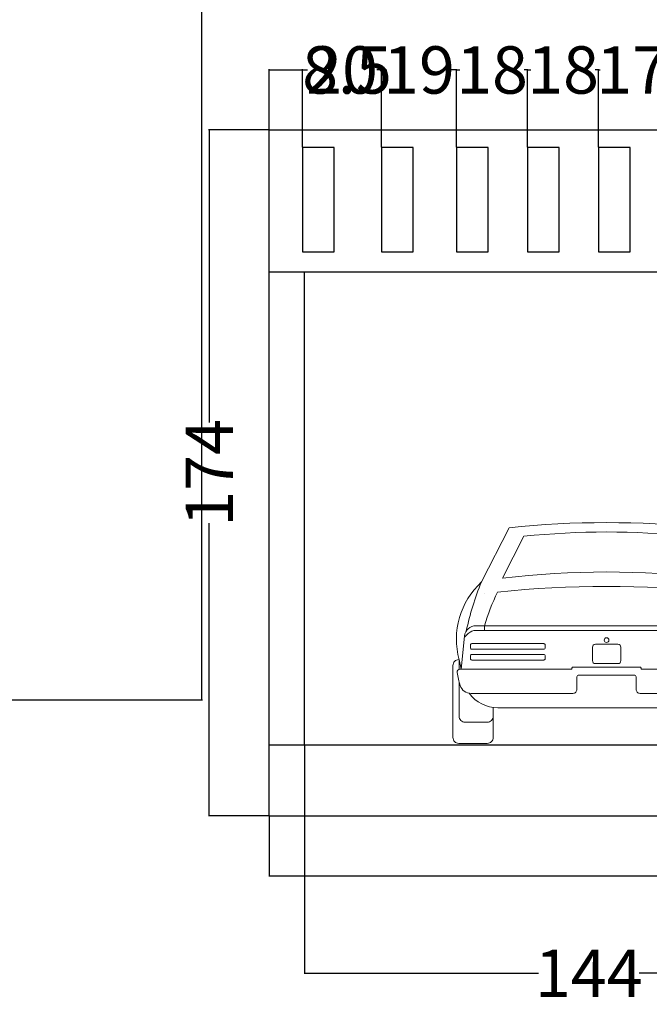
# Model space of a CAD drawing. Units: inches. Extents: x -101 to 786, y 26 to 880.
# Tile 6 of 9: x 379 to 538, y 45 to 295. Entities that reach past the tile are written whole.
import ezdxf

# ---------------------------------------------------------------- set-up
doc = ezdxf.new("R2010")
doc.units = ezdxf.units.IN
doc.header["$MEASUREMENT"] = 0
for name, color, linetype, lineweight in [('A-ANNO-DIMS', 2, 'Continuous', 18), ('A-ELEV', 7, 'Continuous', 30), ('A-EQPM-VEHC', 9, 'Continuous', 13)]:
    doc.layers.add(name, color=color, linetype=linetype, lineweight=lineweight)
doc.styles.get("Standard").update_dxf_attribs({"font": 'arial.ttf'})
doc.dimstyles.get("Standard").update_dxf_attribs({"dimtxt": 12, "dimasz": 0.18, "dimexe": 0.18, "dimexo": 0.0625, "dimgap": 0.09, "dimtad": 0, "dimdec": 1, "dimzin": 0, "dimdsep": 46, "dimlunit": 3, "dimtxsty": 'Standard', "dimcen": 0.09, "dimadec": 0, "dimazin": 0, "dimtfac": 1, "dimtdec": 1, "dimtofl": 0, "dimtmove": 0, "dimatfit": 3, "dimfxl": 1, "dimtolj": 1, "dimtzin": 0, "dimarcsym": 0})

# ---------------------------------------------------------------- blocks, each defined once
blk = doc.blocks.new('*U16')
for p, q in [((-24.66, 54.68), (-31.66, 40.93)), ((31.66, 40.93), (24.66, 54.68)), ((-30.95, 37.96), (-30.95, 37.96)), ((-37.32, 21.22), (-36.82, 18.83)), ((36.82, 18.83), (37.31, 21.2)), ((-27.55, 9), (27.55, 9))]:
    blk.add_line(p, q)
for points in [[(-20.92, 52.5), (-26.31, 41.89), (-26.31, 41.89, -0.059427), (26.31, 41.89), (20.92, 52.5, 0.05217)], [(-34.12, 25.29), (-15.92, 25.29, -0.414214), (-15.55, 24.92), (-15.55, 24.24, -0.414214), (-15.92, 23.87), (-34.12, 23.87, -0.414214), (-34.49, 24.24), (-34.49, 24.92, -0.414214)], [(-2.82, 25.12), (2.9, 25.12, -0.414214), (3.64, 24.38), (3.64, 20.97, -0.414214), (2.9, 20.23), (-2.82, 20.23, -0.414214), (-3.56, 20.97), (-3.56, 24.38, -0.414214)], [(34.12, 25.29), (15.92, 25.29, 0.414214), (15.55, 24.92), (15.55, 24.24, 0.414214), (15.92, 23.87), (34.12, 23.87, 0.414214), (34.49, 24.24), (34.49, 24.92, 0.414214)], [(-34.12, 22.54), (-15.92, 22.54, -0.414214), (-15.55, 22.17), (-15.55, 21.49, -0.414214), (-15.92, 21.12), (-34.12, 21.12, -0.414214), (-34.49, 21.49), (-34.49, 22.17, -0.414214)], [(34.12, 22.54), (15.92, 22.54, 0.414214), (15.55, 22.17), (15.55, 21.49, 0.414214), (15.92, 21.12), (34.12, 21.12, 0.414214), (34.49, 21.49), (34.49, 22.17, 0.414214)], [(-7.5, 16.83, -0.414214), (-7, 17.33), (7, 17.33, -0.414214), (7.5, 16.83), (7.5, 13.67, 0.414214), (8.5, 12.67), (34.29, 12.67, 0.322734), (37.1, 14.69, 0.029256), (37.41, 15.83), (37.84, 17.94, 0.475639), (37.12, 18.83), (9, 18.83, -0.414214), (8.75, 19.08, 0.414214), (8.5, 19.33), (-8.5, 19.33, 0.414214), (-8.75, 19.08, -0.414214), (-9, 18.83), (-37.12, 18.83, 0.475639), (-37.84, 17.94), (-37.41, 15.83, 0.029158), (-37.1, 14.7, 0.322842), (-34.29, 12.67), (-8.5, 12.67, 0.414214), (-7.5, 13.67)]]:
    blk.add_lwpolyline(points, format="xyb", close=True)
for points in [[(30.95, 28.64), (30.95, 29.82, 0.037308), (27.62, 38.34, 0.052989), (-27.62, 38.34, 0.037308), (-30.95, 29.82), (-30.95, 28.64)], [(-36.82, 18.83), (-35.99, 27.2, -0.380946), (-33.05, 29.82), (33.04, 29.82, -0.380474), (35.98, 27.2), (36.82, 18.83)], [(-36.02, 26.89), (-35.02, 27.89, -0.184023), (-33.05, 28.64), (33.05, 28.64, -0.184023), (35.02, 27.89), (36.02, 26.89)], [(-28.73, 9.08), (-28.73, 1.48, -0.414214), (-30.21, 0), (-37.44, 0, -0.414214), (-38.92, 1.48), (-38.92, 19.74, -0.414214), (-37.44, 21.22), (-37.32, 21.22)], [(28.67, 9.07), (28.67, 1.48, 0.414214), (30.15, 0), (37.38, 0, 0.414214), (38.86, 1.48), (38.86, 19.74, 0.414214), (37.38, 21.22), (37.32, 21.22)], [(-37.32, 15.44), (-37.32, 6.85, 0.414214), (-35.84, 5.37), (-30.21, 5.37, 0.414214), (-28.73, 6.85), (-28.73, 9.08)], [(37.32, 15.44), (37.32, 6.85, -0.414214), (35.84, 5.37), (30.21, 5.37, -0.414214), (28.73, 6.85), (28.73, 9.08)]]:
    blk.add_lwpolyline(points, format="xyb")
for points in [[(-37.32, 21.22), (-37.32, 18.8)], [(37.32, 21.22), (37.32, 18.8)]]:
    blk.add_lwpolyline(points)
blk.add_circle((0, 26.18), 0.596)
for centre, radius, start, end in [((0, -181.13), 237.1, 84.03, 95.97), ((-18.4, 26.45), 19.63, 132.4835, 195.4658), ((30.86, 14.66), 67.81, 157.2124, 168.2366), ((18.26, 26.38), 19.77, 344.8595, 47.3598), ((-31.75, 14.41), 68.72, 11.827, 22.6625), ((-27.55, 17.88), 8.88, 215.5776, 270.0028), ((27.55, 17.88), 8.88, 270.0028, 324.3999)]:
    blk.add_arc(centre, radius, start, end)
blk = doc.blocks.new('PARAPET-PANEL-8')
blk.add_lwpolyline([(0, 0), (8, 0), (8, 26.5), (0, 26.5)], close=True)
blk = doc.blocks.new('*D80')
at = {"layer": 'A-ANNO-DIMS', "color": 0, "lineweight": -2, "transparency": 16777216}
for p, q in [((323.57, 781.8), (424.94, 781.8)), ((424.76, 781.62), (424.76, 472.49)), ((424.76, 122.52), (424.76, 431.66)), ((323.57, 122.34), (424.94, 122.34))]:
    blk.add_line(p, q, dxfattribs=at)
at = {"layer": 'A-ANNO-DIMS', "color": 0, "transparency": 16777216}
for points in [[(424.73, 781.62), (424.79, 781.62), (424.76, 781.8)], [(424.73, 122.52), (424.79, 122.52), (424.76, 122.34)]]:
    blk.add_solid(points, dxfattribs=at)
at = {"layer": 'Defpoints', "color": 0, "transparency": 16777216}
for p in [(323.51, 781.8), (424.76, 781.8), (323.51, 122.34)]:
    blk.add_point(p, dxfattribs=at)
at = {"layer": 'A-ANNO-DIMS', "color": 0, "transparency": 16777216, "insert": (424.76, 452.07), "char_height": 12, "attachment_point": 5, "rotation": 90}
blk.add_mtext('\\A1;659.5', dxfattribs=at)
blk = doc.blocks.new('*D89')
at = {"layer": 'A-ANNO-DIMS', "color": 0, "lineweight": -2, "transparency": 16777216}
for p, q in [((441.81, 92.86), (441.81, 77.59)), ((741.81, 92.86), (741.81, 77.59)), ((441.99, 77.77), (578.49, 77.77)), ((741.63, 77.77), (605.13, 77.77))]:
    blk.add_line(p, q, dxfattribs=at)
at = {"layer": 'A-ANNO-DIMS', "color": 0, "transparency": 16777216}
for points in [[(441.99, 77.8), (441.99, 77.74), (441.81, 77.77)], [(741.63, 77.8), (741.63, 77.74), (741.81, 77.77)]]:
    blk.add_solid(points, dxfattribs=at)
at = {"layer": 'Defpoints', "color": 0, "transparency": 16777216}
for p in [(441.81, 92.92), (741.81, 92.92), (441.81, 77.77)]:
    blk.add_point(p, dxfattribs=at)
at = {"layer": 'A-ANNO-DIMS', "color": 0, "transparency": 16777216, "insert": (591.81, 77.77), "char_height": 12, "attachment_point": 5}
blk.add_mtext('\\A1;300', dxfattribs=at)
blk = doc.blocks.new('*D90')
at = {"layer": 'A-ANNO-DIMS', "color": 0, "lineweight": -2, "transparency": 16777216}
for p, q in [((441.81, 266.99), (441.81, 282.25)), ((450.31, 262.49), (450.31, 282.25)), ((441.99, 282.07), (450.13, 282.07)), ((450.31, 282.07), (450.49, 282.07))]:
    blk.add_line(p, q, dxfattribs=at)
at = {"layer": 'A-ANNO-DIMS', "color": 0, "transparency": 16777216}
for points in [[(441.99, 282.1), (441.99, 282.04), (441.81, 282.07)], [(450.13, 282.1), (450.13, 282.04), (450.31, 282.07)]]:
    blk.add_solid(points, dxfattribs=at)
at = {"layer": 'Defpoints', "color": 0, "transparency": 16777216}
for p in [(450.31, 282.07), (441.81, 266.92), (450.31, 262.42)]:
    blk.add_point(p, dxfattribs=at)
at = {"layer": 'A-ANNO-DIMS', "color": 0, "transparency": 16777216, "insert": (461.56, 282.07), "char_height": 12, "attachment_point": 5}
blk.add_mtext('\\A1;8.5', dxfattribs=at)
blk = doc.blocks.new('*D91')
at = {"layer": 'A-ANNO-DIMS', "color": 0, "lineweight": -2, "transparency": 16777216}
for p, q in [((450.31, 262.49), (450.31, 282.25)), ((470.31, 262.49), (470.31, 282.25)), ((450.49, 282.07), (451.55, 282.07)), ((470.13, 282.07), (469.08, 282.07))]:
    blk.add_line(p, q, dxfattribs=at)
at = {"layer": 'A-ANNO-DIMS', "color": 0, "transparency": 16777216}
for points in [[(450.49, 282.1), (450.49, 282.04), (450.31, 282.07)], [(470.13, 282.1), (470.13, 282.04), (470.31, 282.07)]]:
    blk.add_solid(points, dxfattribs=at)
at = {"layer": 'Defpoints', "color": 0, "transparency": 16777216}
for p in [(470.31, 282.07), (450.31, 262.42), (470.31, 262.42)]:
    blk.add_point(p, dxfattribs=at)
at = {"layer": 'A-ANNO-DIMS', "color": 0, "transparency": 16777216, "insert": (460.31, 282.07), "char_height": 12, "attachment_point": 5}
blk.add_mtext('\\A1;20', dxfattribs=at)
blk = doc.blocks.new('*D92')
at = {"layer": 'A-ANNO-DIMS', "color": 0, "lineweight": -2, "transparency": 16777216}
for p, q in [((470.31, 262.49), (470.31, 282.25)), ((489.31, 262.49), (489.31, 282.25)), ((470.49, 282.07), (471.68, 282.07)), ((489.13, 282.07), (487.94, 282.07))]:
    blk.add_line(p, q, dxfattribs=at)
at = {"layer": 'A-ANNO-DIMS', "color": 0, "transparency": 16777216}
for points in [[(470.49, 282.1), (470.49, 282.04), (470.31, 282.07)], [(489.13, 282.1), (489.13, 282.04), (489.31, 282.07)]]:
    blk.add_solid(points, dxfattribs=at)
at = {"layer": 'Defpoints', "color": 0, "transparency": 16777216}
for p in [(489.31, 282.07), (470.31, 262.42), (489.31, 262.42)]:
    blk.add_point(p, dxfattribs=at)
at = {"layer": 'A-ANNO-DIMS', "color": 0, "transparency": 16777216, "insert": (479.81, 282.07), "char_height": 12, "attachment_point": 5}
blk.add_mtext('\\A1;19', dxfattribs=at)
blk = doc.blocks.new('*D93')
at = {"layer": 'A-ANNO-DIMS', "color": 0, "lineweight": -2, "transparency": 16777216}
for p, q in [((489.31, 262.49), (489.31, 282.25)), ((507.31, 262.49), (507.31, 282.25)), ((489.49, 282.07), (490.18, 282.07)), ((507.13, 282.07), (506.44, 282.07))]:
    blk.add_line(p, q, dxfattribs=at)
at = {"layer": 'A-ANNO-DIMS', "color": 0, "transparency": 16777216}
for points in [[(489.49, 282.1), (489.49, 282.04), (489.31, 282.07)], [(507.13, 282.1), (507.13, 282.04), (507.31, 282.07)]]:
    blk.add_solid(points, dxfattribs=at)
at = {"layer": 'Defpoints', "color": 0, "transparency": 16777216}
for p in [(507.31, 282.07), (489.31, 262.42), (507.31, 262.42)]:
    blk.add_point(p, dxfattribs=at)
at = {"layer": 'A-ANNO-DIMS', "color": 0, "transparency": 16777216, "insert": (498.31, 282.07), "char_height": 12, "attachment_point": 5}
blk.add_mtext('\\A1;18', dxfattribs=at)
blk = doc.blocks.new('*D94')
at = {"layer": 'A-ANNO-DIMS', "color": 0, "lineweight": -2, "transparency": 16777216}
for p, q in [((507.31, 262.49), (507.31, 282.25)), ((525.31, 262.49), (525.31, 282.25)), ((507.49, 282.07), (508.18, 282.07)), ((525.13, 282.07), (524.44, 282.07))]:
    blk.add_line(p, q, dxfattribs=at)
at = {"layer": 'A-ANNO-DIMS', "color": 0, "transparency": 16777216}
for points in [[(507.49, 282.1), (507.49, 282.04), (507.31, 282.07)], [(525.13, 282.1), (525.13, 282.04), (525.31, 282.07)]]:
    blk.add_solid(points, dxfattribs=at)
at = {"layer": 'Defpoints', "color": 0, "transparency": 16777216}
for p in [(525.31, 282.07), (507.31, 262.42), (525.31, 262.42)]:
    blk.add_point(p, dxfattribs=at)
at = {"layer": 'A-ANNO-DIMS', "color": 0, "transparency": 16777216, "insert": (516.31, 282.07), "char_height": 12, "attachment_point": 5}
blk.add_mtext('\\A1;18', dxfattribs=at)
blk = doc.blocks.new('*D95')
at = {"layer": 'A-ANNO-DIMS', "color": 0, "lineweight": -2, "transparency": 16777216}
for p, q in [((525.31, 262.49), (525.31, 282.25)), ((542.31, 262.49), (542.31, 282.25)), ((525.49, 282.07), (525.69, 282.07)), ((542.13, 282.07), (541.93, 282.07))]:
    blk.add_line(p, q, dxfattribs=at)
at = {"layer": 'A-ANNO-DIMS', "color": 0, "transparency": 16777216}
for points in [[(525.49, 282.1), (525.49, 282.04), (525.31, 282.07)], [(542.13, 282.1), (542.13, 282.04), (542.31, 282.07)]]:
    blk.add_solid(points, dxfattribs=at)
at = {"layer": 'Defpoints', "color": 0, "transparency": 16777216}
for p in [(542.31, 282.07), (525.31, 262.42), (542.31, 262.42)]:
    blk.add_point(p, dxfattribs=at)
at = {"layer": 'A-ANNO-DIMS', "color": 0, "transparency": 16777216, "insert": (533.81, 282.07), "char_height": 12, "attachment_point": 5}
blk.add_mtext('\\A1;17', dxfattribs=at)
blk = doc.blocks.new('*D106')
at = {"layer": 'A-ANNO-DIMS', "color": 0, "lineweight": -2, "transparency": 16777216}
for p, q in [((441.75, 266.92), (426.48, 266.92)), ((426.66, 266.74), (426.66, 192.68)), ((426.66, 93.1), (426.66, 167.17)), ((441.75, 92.92), (426.48, 92.92))]:
    blk.add_line(p, q, dxfattribs=at)
at = {"layer": 'A-ANNO-DIMS', "color": 0, "transparency": 16777216}
for points in [[(426.63, 266.74), (426.69, 266.74), (426.66, 266.92)], [(426.63, 93.1), (426.69, 93.1), (426.66, 92.92)]]:
    blk.add_solid(points, dxfattribs=at)
at = {"layer": 'Defpoints', "color": 0, "transparency": 16777216}
for p in [(426.66, 266.92), (441.81, 266.92), (441.81, 92.92)]:
    blk.add_point(p, dxfattribs=at)
at = {"layer": 'A-ANNO-DIMS', "color": 0, "transparency": 16777216, "insert": (426.66, 179.92), "char_height": 12, "attachment_point": 5, "rotation": 90}
blk.add_mtext('\\A1;174', dxfattribs=at)
blk = doc.blocks.new('*D115')
at = {"layer": 'A-ANNO-DIMS', "color": 0, "lineweight": -2, "transparency": 16777216}
for p, q in [((450.81, 110.86), (450.81, 52.87)), ((594.81, 110.86), (594.81, 52.87)), ((450.99, 53.05), (510.05, 53.05)), ((594.63, 53.05), (535.57, 53.05))]:
    blk.add_line(p, q, dxfattribs=at)
at = {"layer": 'A-ANNO-DIMS', "color": 0, "transparency": 16777216}
for points in [[(450.99, 53.08), (450.99, 53.02), (450.81, 53.05)], [(594.63, 53.08), (594.63, 53.02), (594.81, 53.05)]]:
    blk.add_solid(points, dxfattribs=at)
at = {"layer": 'Defpoints', "color": 0, "transparency": 16777216}
for p in [(450.81, 110.92), (594.81, 110.92), (594.81, 53.05)]:
    blk.add_point(p, dxfattribs=at)
at = {"layer": 'A-ANNO-DIMS', "color": 0, "transparency": 16777216, "insert": (522.81, 53.05), "char_height": 12, "attachment_point": 5}
blk.add_mtext('\\A1;144', dxfattribs=at)

msp = doc.modelspace()

# ---------------------------------------------------------------- linework, layer by layer
at = {"layer": 'A-ELEV'}
for p, q in [((441.8117, 92.9238), (441.8117, 266.9238)), ((441.8117, 266.9238), (741.8117, 266.9238)), ((441.8117, 230.9238), (741.8117, 230.9238)), ((450.8117, 110.9238), (450.8117, 230.9238)), ((441.8117, 110.9238), (741.8117, 110.9238)), ((441.8117, 92.9238), (741.8117, 92.9238))]:
    msp.add_line(p, q, dxfattribs=at)

# ---------------------------------------------------------------- block references
for p in [(450.312, 235.924), (470.312, 235.924), (489.312, 235.924), (507.312, 235.924), (525.312, 235.924)]:
    msp.add_blockref('PARAPET-PANEL-8', p, dxfattribs=at)
at = {"layer": 'A-EQPM-VEHC'}
msp.add_blockref('*U16', (527.3117, 111.3367), dxfattribs=at)

# ---------------------------------------------------------------- dimensions: what is measured, and where the dimension line sits
at = {"layer": 'A-ANNO-DIMS'}
for base, p1, p2, angle, override, picture, middle in [((424.7579, 781.8033), (323.5071, 122.3446), (323.5071, 781.8033), 90, {"dimdec": 1, "dimlfac": 1, "dimrnd": 0, "dimzin": 0, "dimdsep": 46, "dimlunit": 2}, '*D80', (424.7579, 452.0739)), ((426.6617, 266.9238), (441.8117, 92.9238), (441.8117, 266.9238), 90, {"dimdec": 0, "dimlfac": 1, "dimrnd": 0, "dimzin": 0, "dimdsep": 46, "dimlunit": 2}, '*D106', (426.6617, 179.9238)), ((441.8117, 77.7738), (741.8117, 92.9238), (441.8117, 92.9238), 180, {"dimdec": 0, "dimlfac": 1, "dimrnd": 0, "dimzin": 0, "dimdsep": 46, "dimlunit": 2}, '*D89', (591.8117, 77.7738))]:
    dim = msp.add_linear_dim(base=base, p1=p1, p2=p2, angle=angle, dimstyle='Standard', override=override, dxfattribs=at)
    dim.commit()
    dim.dimension.update_dxf_attribs({"geometry": picture, "text_midpoint": middle})
for base, p1, p2, override, picture, middle in [((450.3117, 282.0738), (441.8117, 266.9238), (450.3117, 262.4238), {"dimdec": 1, "dimlfac": 1, "dimrnd": 0, "dimzin": 0, "dimdsep": 46, "dimlunit": 2}, '*D90', (461.5585, 282.0738)), ((470.3117, 282.0738), (450.3117, 262.4238), (470.3117, 262.4238), {"dimdec": 0, "dimlfac": 1, "dimrnd": 0, "dimzin": 0, "dimdsep": 46, "dimlunit": 2}, '*D91', (460.3117, 282.0738)), ((489.3117, 282.0738), (470.3117, 262.4238), (489.3117, 262.4238), {"dimdec": 0, "dimlfac": 1, "dimrnd": 0, "dimzin": 0, "dimdsep": 46, "dimlunit": 2}, '*D92', (479.8117, 282.0738)), ((507.3117, 282.0738), (489.3117, 262.4238), (507.3117, 262.4238), {"dimdec": 0, "dimlfac": 1, "dimrnd": 0, "dimzin": 0, "dimdsep": 46, "dimlunit": 2}, '*D93', (498.3117, 282.0738)), ((525.3117, 282.0738), (507.3117, 262.4238), (525.3117, 262.4238), {"dimdec": 0, "dimlfac": 1, "dimrnd": 0, "dimzin": 0, "dimdsep": 46, "dimlunit": 2}, '*D94', (516.3117, 282.0738)), ((542.3117, 282.0738), (525.3117, 262.4238), (542.3117, 262.4238), {"dimdec": 0, "dimlfac": 1, "dimrnd": 0, "dimzin": 0, "dimdsep": 46, "dimlunit": 2}, '*D95', (533.8117, 282.0738)), ((594.8117, 53.0498), (450.8117, 110.9238), (594.8117, 110.9238), {"dimdec": 0, "dimlfac": 1, "dimrnd": 0, "dimzin": 0, "dimdsep": 46, "dimlunit": 2}, '*D115', (522.8117, 53.0498))]:
    dim = msp.add_linear_dim(base=base, p1=p1, p2=p2, dimstyle='Standard', override=override, dxfattribs=at)
    dim.commit()
    dim.dimension.update_dxf_attribs({"geometry": picture, "text_midpoint": middle})

doc.saveas('drawing.dxf')
